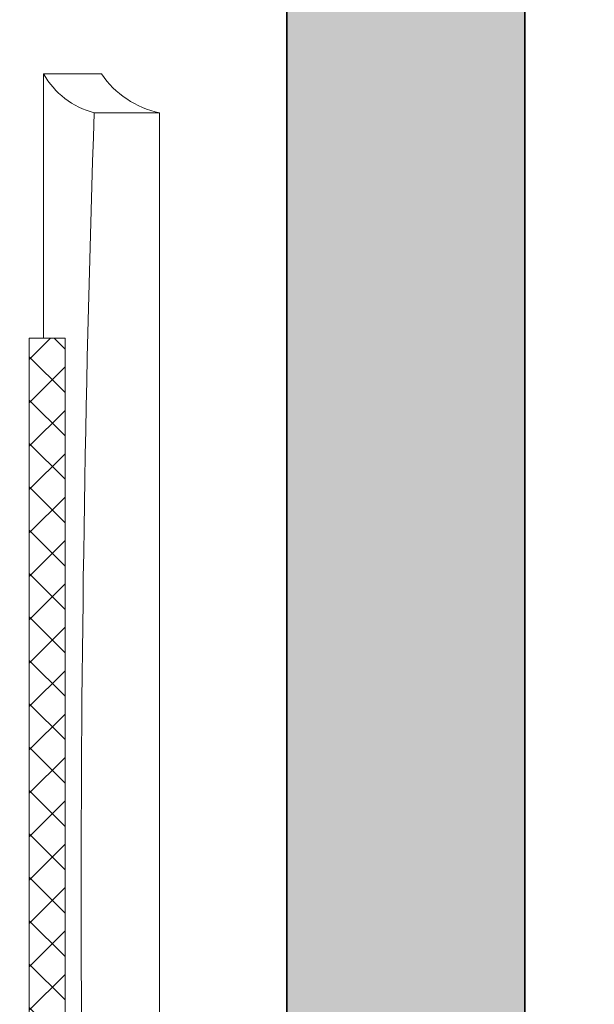
# Model space of a CAD drawing. Units: inches. Extents: x 2083 to 3317, y 1141 to 2115.
# Tile 243 of 256: x 3108 to 3130, y 1327 to 1365. Entities that reach past the tile are written whole.
import ezdxf

# ---------------------------------------------------------------- set-up
doc = ezdxf.new("R2010")
doc.units = ezdxf.units.IN
for name, color, linetype, lineweight in [('A-ANNO-DIMS', 2, 'Continuous', 18), ('A-FURN', 8, 'Continuous', 18), ('A-WALL', 7, 'Continuous', 35), ('www.cadblocksfree.com', 7, 'Continuous', 9)]:
    doc.layers.add(name, color=color, linetype=linetype, lineweight=lineweight)
doc.layers.add('A-WALL-PATT', color=251, linetype='Continuous', lineweight=13, true_color=0x636466)
doc.styles.get("Standard").update_dxf_attribs({"font": 'arial.ttf'})
doc.dimstyles.new('ISO-25', dxfattribs={"dimtxt": 12, "dimasz": 12, "dimexe": 1.25, "dimexo": 0.625, "dimtad": 1, "dimlunit": 3, "dimtxsty": 'Standard', "dimcen": 2.5, "dimadec": 0, "dimazin": 0, "dimtfac": 1, "dimtmove": 0, "dimatfit": 3, "dimfxl": 1, "dimarcsym": 0})

# ---------------------------------------------------------------- blocks, each defined once
blk = doc.blocks.new('bed')
at = {"layer": 'www.cadblocksfree.com', "ltscale": 0.2}
h = blk.add_hatch(dxfattribs=at)
h.set_pattern_fill('ANSI37,_O', color=256, scale=0.393701)
h.set_pattern_definition([(45, (2420.7222, -262.9689), (-0.8838835, 0.8838835), []), (135, (2420.7222, -262.9689), (-0.8838835, -0.8838835), [])])
h.paths.add_polyline_path([(3417.573, 1472.402), (3372.192, 1472.402), (3372.192, 1470.941), (3417.573, 1470.941)])
for p, q in [((3363.002, 1473.586), (3363.002, 1476.249)), ((3372.192, 1472.402), (3417.573, 1472.402)), ((3372.192, 1470.941), (3372.192, 1472.402)), ((3372.192, 1470.941), (3417.573, 1470.941))]:
    blk.add_line(p, q, dxfattribs=at)
for points in [[(3426.763, 1476.249), (3363.002, 1476.249)], [(3361.418, 1473.886), (3361.418, 1471.524), (3372.192, 1471.524)]]:
    blk.add_lwpolyline(points, dxfattribs=at)
for centre, radius, start, end in [((3359.334, 1476.997), 3.744, 303.8271, 348.4775), ((3359.844, 1474.373), 3.255, 298.9176, 345.9939), ((3394.883, 2431.358), 958.303, 268.093559, 271.906441)]:
    blk.add_arc(centre, radius, start, end, dxfattribs=at)
blk = doc.blocks.new('*D9')
at = {"layer": 'A-ANNO-DIMS', "color": 0, "lineweight": -2, "transparency": 16777216}
for p, q in [((3127.585, 1486.761), (3190.403, 1486.761)), ((3189.153, 1474.761), (3189.153, 1275.261)), ((3127.585, 1263.261), (3190.403, 1263.261))]:
    blk.add_line(p, q, dxfattribs=at)
at = {"layer": 'A-ANNO-DIMS', "color": 0, "transparency": 16777216}
for points in [[(3187.153, 1474.761), (3191.153, 1474.761), (3189.153, 1486.761)], [(3187.153, 1275.261), (3191.153, 1275.261), (3189.153, 1263.261)]]:
    blk.add_solid(points, dxfattribs=at)
at = {"layer": 'Defpoints', "color": 0, "transparency": 16777216}
for p in [(3126.96, 1486.761), (3126.96, 1263.261), (3189.153, 1263.261)]:
    blk.add_point(p, dxfattribs=at)
at = {"layer": 'A-ANNO-DIMS', "color": 0, "transparency": 16777216, "insert": (3182.401, 1375.011), "char_height": 12, "attachment_point": 5, "rotation": 90}
blk.add_mtext('18\'-7.5"', dxfattribs=at)
blk = doc.blocks.new('*D35')
at = {"layer": 'A-ANNO-DIMS', "color": 0, "lineweight": -2, "transparency": 16777216}
for p, q in [((3127.585, 2020.761), (3180.56, 2020.761)), ((3179.31, 1275.261), (3179.31, 2008.761)), ((3127.585, 1263.261), (3180.56, 1263.261))]:
    blk.add_line(p, q, dxfattribs=at)
at = {"layer": 'A-ANNO-DIMS', "color": 0, "transparency": 16777216}
for points in [[(3177.31, 2008.761), (3181.31, 2008.761), (3179.31, 2020.761)], [(3177.31, 1275.261), (3181.31, 1275.261), (3179.31, 1263.261)]]:
    blk.add_solid(points, dxfattribs=at)
at = {"layer": 'Defpoints', "color": 0, "transparency": 16777216}
for p in [(3126.96, 2020.761), (3179.31, 2020.761), (3126.96, 1263.261)]:
    blk.add_point(p, dxfattribs=at)
at = {"layer": 'A-ANNO-DIMS', "color": 0, "transparency": 16777216, "insert": (3172.476, 1642.011), "char_height": 12, "attachment_point": 5, "rotation": 90}
blk.add_mtext('63\'-1 1/2"', dxfattribs=at)

msp = doc.modelspace()

# ---------------------------------------------------------------- hatches: boundary and pattern name
at = {"layer": 'A-WALL-PATT'}
h = msp.add_hatch(color=256, dxfattribs=at)
h.dxf.hatch_style = 1
h.paths.add_polyline_path([(3126.96, 2020.761), (2748.96, 2020.761), (2604.96, 2020.761), (2226.96, 2020.761), (2226.96, 1702.761), (2466.96, 1702.761), (2466.96, 1582.761), (2418.96, 1582.761), (2418.96, 1477.761), (2226.96, 1477.761), (2226.96, 1263.261), (2544.96, 1263.261), (2544.96, 1411.761), (2604.96, 1411.761), (2685.96, 1411.761), (2685.96, 1420.761), (2604.96, 1420.761), (2604.96, 1573.761), (2604.96, 1702.761), (2604.96, 2011.761), (2748.96, 2011.761), (2748.96, 1702.761), (2862.96, 1702.761), (2862.96, 1621.761), (2871.96, 1621.761), (2871.96, 1702.761), (2883.96, 1702.761), (2883.96, 1706.939, -0.026459), (2883.96, 1711.761), (2757.96, 1711.761), (2757.96, 1807.761), (2787.96, 1807.761), (2787.96, 1812.261), (2757.96, 1812.261), (2757.96, 2011.761), (2877.96, 2011.761), (2877.96, 1812.261), (2847.96, 1812.261), (2847.96, 1807.761), (2889.836, 1807.761), (2889.836, 1812.261), (2882.46, 1812.261), (2882.46, 2011.761), (3117.96, 2011.761), (3117.96, 1812.261), (2937.836, 1812.261), (2937.836, 1807.761), (2995.71, 1807.761), (2995.71, 1796.118), (3000.21, 1796.118), (3000.21, 1807.761), (3117.96, 1807.761), (3117.96, 1711.761), (3000.21, 1711.761), (3000.21, 1760.118), (2998.573, 1760.118, -0.020711), (2995.71, 1760.118), (2995.71, 1711.761), (2931.96, 1711.761), (2931.96, 1702.761), (3126.96, 1702.761)])
h.paths.add_polyline_path([(2471.46, 2011.761), (2471.46, 1810.011), (2462.717, 1810.011), (2462.717, 1805.511), (2505.96, 1805.511), (2505.96, 1810.011), (2475.96, 1810.011), (2475.96, 2011.761), (2595.96, 2011.761), (2595.96, 1810.011), (2565.96, 1810.011), (2565.96, 1805.511), (2595.96, 1805.511), (2595.96, 1711.761), (2235.96, 1711.761), (2235.96, 1805.511), (2353.71, 1805.511), (2353.71, 1796.054), (2358.21, 1796.054), (2358.21, 1805.511), (2414.717, 1805.511), (2414.717, 1810.011), (2235.96, 1810.011), (2235.96, 2011.761)], flags=16)
h.paths.add_polyline_path([(2270.205, 1994.61), (2270.205, 1970.61), (2246.205, 1970.61), (2246.205, 1994.61)], flags=0)
edge = h.paths.add_edge_path(flags=0)
edge.add_ellipse((2332.027, 1899.798), major_axis=(-3.043, 3.043), ratio=0.168252, start_angle=-161.3322, end_angle=-156.3071, ccw=False)
edge.add_ellipse((2333.082, 1898.744), major_axis=(-1.055, 1.055), ratio=0.453532, start_angle=-123.371, end_angle=-94.1591)
edge = h.paths.add_edge_path(flags=0)
edge.add_ellipse((2332.027, 1968.876), major_axis=(3.043, 3.043), ratio=0.168252, start_angle=18.6678, end_angle=23.6929)
edge.add_spline(control_points=[(2332.926, 1970.691), (2332.227, 1970.336), (2330.894, 1969.659), (2328.413, 1970.932), (2327.204, 1967.749), (2324.71, 1969.956), (2322.533, 1967.012), (2320.013, 1971.296), (2317.68, 1968.158), (2316.041, 1967.102), (2315.427, 1966.81)], knot_values=[0, 0, 0, 0, 2.267059, 4.324559, 6.685584, 8.878641, 11.121502, 14.300359, 17.755284, 19.732645, 19.732645, 19.732645, 19.732645], degree=3, periodic=0)
edge.add_ellipse((2332.027, 1968.876), major_axis=(3.043, 3.043), ratio=0.168252, start_angle=18.6678, end_angle=23.6929, ccw=False)
edge.add_ellipse((2333.082, 1969.931), major_axis=(1.055, 1.055), ratio=0.453532, start_angle=56.629, end_angle=85.8409, ccw=False)
edge = h.paths.add_edge_path(flags=0)
edge.add_spline(control_points=[(2296.428, 1967.988), (2293.628, 1965.336), (2287.704, 1959.727), (2299.744, 1949.996), (2294.533, 1935.669), (2290.573, 1920.604), (2293.394, 1909.974), (2296.185, 1904.967)], knot_values=[0.099185, 0.099185, 0.099185, 0.099185, 0.345301, 0.619822, 0.982653, 1.386093, 1.810555, 1.810555, 1.810555, 1.810555], degree=3, periodic=0)
edge.add_spline(control_points=[(2296.185, 1904.967), (2297.384, 1902.619), (2298.001, 1901.949), (2298.553, 1901.468)], knot_values=[0.006246, 0.006246, 0.006246, 0.006246, 0.055476, 0.055476, 0.055476, 0.055476], degree=3, periodic=0)
edge.add_spline(control_points=[(2298.553, 1901.468), (2297.259, 1900.923), (2295.225, 1900.232), (2293.06, 1900.614), (2292.101, 1900.788), (2292.09, 1900.791)], knot_values=[0.312835, 0.312835, 0.312835, 0.312835, 0.40178, 0.474987, 0.475903, 0.475903, 0.475903, 0.475903], degree=3, periodic=0)
edge.add_arc((2292.794, 1904.664), 3.937, 215.4209, 259.6982, ccw=False)
edge.add_spline(control_points=[(2289.585, 1902.382), (2289.477, 1902.535), (2289.368, 1902.688), (2289.261, 1902.841)], knot_values=[0.102872, 0.102872, 0.102872, 0.102872, 0.116896, 0.116896, 0.116896, 0.116896], degree=3, periodic=0)
edge.add_spline(control_points=[(2289.261, 1902.841), (2288.687, 1902.55), (2287.64, 1902.02), (2285.881, 1901.874), (2283.853, 1901.504), (2281.72, 1899.711), (2278.467, 1899.493), (2276.157, 1901.883), (2272.259, 1899.804), (2267.778, 1901.843), (2262.244, 1900.184), (2257.415, 1901.782), (2254.318, 1900.726), (2253.178, 1900.337)], knot_values=[0, 0, 0, 0, 1.907977, 3.477176, 5.261074, 7.972851, 11.680248, 13.717921, 16.939592, 22.789562, 27.502503, 33.595215, 37.145618, 37.145618, 37.145618, 37.145618], degree=3, periodic=0)
edge.add_line((2253.178, 1900.337), (2250.244, 1902.841))
edge.add_line((2250.244, 1902.841), (2250.244, 1965.833))
edge.add_line((2250.244, 1965.833), (2253.178, 1968.337))
edge.add_spline(control_points=[(2253.178, 1968.337), (2254.318, 1967.948), (2257.415, 1966.892), (2262.244, 1968.49), (2267.778, 1966.831), (2271.527, 1968.537), (2273.876, 1967.828), (2274.207, 1967.728)], knot_values=[0, 0, 0, 0, 0.09018, 0.244935, 0.364644, 0.513233, 0.537855, 0.537855, 0.537855, 0.537855], degree=3, periodic=0)
edge.add_arc((2274.353, 1963.793), 3.937, 72.0511, 92.1279, ccw=False)
edge.add_arc((2281.297, 1985.23), 18.596, 252.0511, 288.5657)
edge.add_arc((2292.317, 1956.029), 12.646, 71.0268, 113.7782, ccw=False)
edge = h.paths.add_edge_path(flags=0)
edge.add_spline(control_points=[(2274.899, 1951.856), (2275.066, 1951.617), (2275.233, 1951.377), (2275.398, 1951.136)], knot_values=[1.409916, 1.409916, 1.409916, 1.409916, 1.43159, 1.43159, 1.43159, 1.43159], degree=3, periodic=0)
edge.add_spline(control_points=[(2275.398, 1951.136), (2275.792, 1950.562), (2276.179, 1949.984), (2276.546, 1949.397)], knot_values=[1.358238, 1.358238, 1.358238, 1.358238, 1.409916, 1.409916, 1.409916, 1.409916], degree=3, periodic=0)
edge.add_line((2276.546, 1949.397), (2277.437, 1947.862))
edge.add_spline(control_points=[(2277.437, 1947.862), (2276.304, 1945.673), (2274.64, 1942.427), (2274.632, 1938.094), (2272.799, 1930.852), (2274.356, 1943.897), (2275.948, 1947.923), (2276.546, 1949.397)], knot_values=[0.005632, 0.005632, 0.005632, 0.005632, 0.186014, 0.266002, 0.357087, 0.59639, 0.739732, 0.739732, 0.739732, 0.739732], degree=3, periodic=0)
edge.add_spline(control_points=[(2276.546, 1949.397), (2276.179, 1949.984), (2275.792, 1950.562), (2275.398, 1951.136)], knot_values=[1.358238, 1.358238, 1.358238, 1.358238, 1.409916, 1.409916, 1.409916, 1.409916], degree=3, periodic=0)
edge.add_spline(control_points=[(2275.398, 1951.136), (2274.943, 1950.08), (2274.208, 1948.025), (2273.935, 1944.851), (2272.469, 1937.627), (2273.466, 1945.696), (2274.701, 1951.059), (2274.899, 1951.856)], knot_values=[0.104364, 0.104364, 0.104364, 0.104364, 0.189636, 0.269624, 0.36071, 0.600013, 0.644622, 0.644622, 0.644622, 0.644622], degree=3, periodic=0)
h.paths.add_polyline_path([(2269.168, 1963.128, -0.357527), (2268.171, 1960.976, -0.092561), (2268.171, 1939.436, -0.357527), (2269.168, 1937.285, -0.357527), (2267.016, 1938.282, -0.164785), (2254.686, 1938.282, -0.357527), (2252.534, 1937.285, -0.357527), (2253.531, 1939.436, -0.092561), (2253.531, 1960.976, -0.357527), (2252.534, 1963.128, -0.357527), (2254.686, 1962.131, -0.164785), (2267.016, 1962.131, -0.357527)], flags=0)
h.paths.add_polyline_path([(2248.874, 1967.802), (2248.874, 1957.028), (2249.458, 1957.028), (2249.458, 1911.647), (2248.874, 1911.647), (2248.874, 1900.873), (2246.512, 1900.873, 0.197327), (2244.15, 1902.457), (2244.15, 1966.218, 0.197327), (2246.512, 1967.802)], flags=0)
h.paths.add_polyline_path([(2269.168, 1931.389, -0.357527), (2268.171, 1929.238, -0.092561), (2268.171, 1907.698, -0.357527), (2269.168, 1905.547, -0.357527), (2267.016, 1906.544, -0.164785), (2254.686, 1906.544, -0.357527), (2252.534, 1905.547, -0.357527), (2253.531, 1907.698, -0.092561), (2253.531, 1929.238, -0.357527), (2252.534, 1931.389, -0.357527), (2254.686, 1930.392, -0.164785), (2267.016, 1930.392, -0.357527)], flags=0)
edge = h.paths.add_edge_path(flags=0)
edge.add_spline(control_points=[(2276.197, 1906.724), (2276.168, 1909.029), (2276.114, 1913.372), (2270.598, 1924.925), (2273.905, 1919.013), (2275.922, 1916.262), (2275.475, 1912.402), (2277.258, 1910.381), (2276.696, 1908.225), (2276.646, 1906.813), (2276.618, 1906.008)], knot_values=[0, 0, 0, 0, 8.61026, 16.221274, 18.843057, 23.804898, 27.440828, 29.356102, 31.203478, 33.650687, 33.650687, 33.650687, 33.650687], degree=3, periodic=0)
edge.add_spline(control_points=[(2276.618, 1906.008), (2276.623, 1905.624), (2276.498, 1904.629), (2275.442, 1903.855), (2274.937, 1903.08), (2274.859, 1902.841)], knot_values=[0.156488, 0.156488, 0.156488, 0.156488, 0.184398, 0.231376, 0.250598, 0.250598, 0.250598, 0.250598], degree=3, periodic=0)
edge.add_line((2274.859, 1902.841), (2276.506, 1902.841))
edge.add_spline(control_points=[(2276.506, 1902.841), (2276.788, 1903.085), (2277.665, 1904.125), (2278.25, 1904.341), (2277.654, 1908.527), (2278.156, 1906.228), (2278.1, 1905.286), (2278.847, 1904.069), (2277.857, 1903.415), (2277.874, 1902.991), (2277.904, 1902.841)], knot_values=[0.059574, 0.059574, 0.059574, 0.059574, 0.080753, 0.103741, 0.16972, 0.176036, 0.207137, 0.240474, 0.262341, 0.27366, 0.27366, 0.27366, 0.27366], degree=3, periodic=0)
edge.add_line((2277.904, 1902.841), (2280.03, 1902.841))
edge.add_spline(control_points=[(2280.03, 1902.841), (2279.888, 1903.088), (2279.499, 1903.982), (2280.152, 1905.939), (2278.104, 1909.658), (2279.762, 1907.185), (2280.328, 1904.875), (2280.485, 1903.49), (2281.463, 1903.249), (2281.758, 1902.936), (2281.834, 1902.841)], knot_values=[0.013856, 0.013856, 0.013856, 0.013856, 0.034874, 0.088867, 0.107879, 0.126738, 0.158714, 0.193757, 0.217487, 0.226722, 0.226722, 0.226722, 0.226722], degree=3, periodic=0)
edge.add_spline(control_points=[(2281.834, 1902.841), (2281.788, 1902.827), (2281.647, 1902.783), (2281.396, 1902.859), (2281.088, 1902.985), (2280.721, 1903.061), (2280.333, 1903.026), (2280.125, 1902.899), (2280.03, 1902.841)], knot_values=[0, 0, 0, 0, 0.14413, 0.435517, 0.749276, 1.153046, 1.548371, 1.878348, 1.878348, 1.878348, 1.878348], degree=3, periodic=0)
edge.add_line((2280.03, 1902.841), (2277.904, 1902.841))
edge.add_spline(control_points=[(2277.904, 1902.841), (2277.893, 1902.796), (2277.865, 1902.68), (2277.607, 1902.687), (2277.274, 1902.801), (2276.838, 1902.62), (2276.584, 1902.789), (2276.506, 1902.841)], knot_values=[0, 0, 0, 0, 0.127189, 0.326199, 0.628009, 1.24357, 1.515331, 1.515331, 1.515331, 1.515331], degree=3, periodic=0)
edge.add_line((2276.506, 1902.841), (2274.859, 1902.841))
edge.add_spline(control_points=[(2274.859, 1902.841), (2274.814, 1902.899), (2274.725, 1903.013), (2274.493, 1903.119), (2274.244, 1902.961), (2273.937, 1903.185), (2273.614, 1902.983), (2273.408, 1902.883), (2273.322, 1902.841)], knot_values=[0, 0, 0, 0, 0.21843, 0.436957, 0.687977, 0.990379, 1.398396, 1.69185, 1.69185, 1.69185, 1.69185], degree=3, periodic=0)
edge.add_spline(control_points=[(2273.322, 1902.841), (2273.617, 1903.446), (2274.274, 1904.538), (2276.027, 1904.574), (2276.207, 1906.584), (2276.197, 1906.724)], knot_values=[0.012227, 0.012227, 0.012227, 0.012227, 0.059472, 0.106218, 0.134458, 0.134458, 0.134458, 0.134458], degree=3, periodic=0)
h.paths.add_polyline_path([(2270.776, 1897.79), (2270.776, 1873.79), (2246.776, 1873.79), (2246.776, 1897.79)], flags=0)
h.paths.add_polyline_path([(2353.71, 1760.005), (2353.71, 1760.054), (2358.21, 1760.054, -0.033729)], flags=0)
h.paths.add_polyline_path([(2321.819, 1737.529), (2341.995, 1737.529, -0.414214), (2343.203, 1736.321), (2343.203, 1721.021, -0.414214), (2341.995, 1719.813), (2321.819, 1719.813, -0.414214), (2320.611, 1721.021), (2320.611, 1736.321, -0.414214)], flags=0)
h.paths.add_polyline_path([(2324.235, 1736.321), (2339.579, 1736.321, -0.414214), (2341.995, 1733.905), (2341.995, 1725.45, -0.414214), (2339.579, 1723.034), (2333.681, 1723.034), (2333.845, 1722.045, -0.870646), (2335.425, 1721.826, -0.767327), (2333.923, 1721.423), (2331.291, 1721.423, -0.767327), (2329.788, 1721.826, -0.870646), (2331.368, 1722.045), (2331.533, 1723.034), (2324.235, 1723.034, -0.414214), (2321.819, 1725.45), (2321.819, 1733.905, -0.414214)], flags=0)
h.paths.add_polyline_path([(2570.484, 1928.615), (2589.684, 1928.615), (2590.169, 1928.615), (2590.169, 1904.993), (2570.484, 1904.993)], flags=0)
h.paths.add_polyline_path([(2574.447, 1927.264, -1), (2572.829, 1927.264, -1)], flags=0)
h.paths.add_polyline_path([(2573.09, 1926.941), (2573.925, 1927.776), (2574.148, 1927.553), (2573.313, 1926.718)], flags=0)
h.paths.add_polyline_path([(2578.779, 1919.73, -1), (2571.592, 1919.73, -1)], flags=0)
h.paths.add_polyline_path([(2578.385, 1919.73, -1), (2571.985, 1919.73, -1)], flags=0)
h.paths.add_polyline_path([(2331.596, 1729.476, -1), (2333.618, 1729.476, -1)], flags=0)
h.paths.add_polyline_path([(2578.034, 1927.264, -1), (2576.416, 1927.264, -1)], flags=0)
h.paths.add_polyline_path([(2576.689, 1927.531), (2576.912, 1927.754), (2577.747, 1926.919), (2577.524, 1926.696)], flags=0)
h.paths.add_polyline_path([(2578.139, 1909.86, -1), (2572.232, 1909.86, -1)], flags=0)
h.paths.add_polyline_path([(2577.745, 1909.86, -1), (2572.625, 1909.86, -1)], flags=0)
h.paths.add_polyline_path([(2583.798, 1927.264, -1), (2582.179, 1927.264, -1)], flags=0)
h.paths.add_polyline_path([(2582.719, 1927.754), (2583.554, 1926.919), (2583.331, 1926.696), (2582.496, 1927.531)], flags=0)
h.paths.add_polyline_path([(2582.496, 1927.531), (2582.719, 1927.754), (2583.554, 1926.919), (2583.331, 1926.696)], flags=0)
h.paths.add_polyline_path([(2587.739, 1920.53, -1), (2581.832, 1920.53, -1)], flags=0)
h.paths.add_polyline_path([(2587.345, 1920.53, -1), (2582.225, 1920.53, -1)], flags=0)
h.paths.add_polyline_path([(2587.385, 1927.264, -1), (2585.766, 1927.264, -1)], flags=0)
h.paths.add_polyline_path([(2586.082, 1926.98), (2586.917, 1927.815), (2587.14, 1927.593), (2586.305, 1926.758)], flags=0)
h.paths.add_polyline_path([(2588.379, 1910.66, -1), (2581.192, 1910.66, -1)], flags=0)
h.paths.add_polyline_path([(2587.985, 1910.66, -1), (2581.585, 1910.66, -1)], flags=0)
h.paths.add_polyline_path([(2417.168, 1729.478), (2437.344, 1729.478, -0.414214), (2438.552, 1728.27), (2438.552, 1712.969, -0.414214), (2437.344, 1711.761), (2417.168, 1711.761, -0.414214), (2415.96, 1712.969), (2415.96, 1728.27, -0.414214)], flags=0)
h.paths.add_polyline_path([(2419.584, 1728.27), (2434.928, 1728.27, -0.414214), (2437.344, 1725.854), (2437.344, 1717.398, -0.414214), (2434.928, 1714.983), (2429.029, 1714.983), (2429.194, 1713.994, -0.870646), (2430.774, 1713.775, -0.767327), (2429.271, 1713.372), (2426.64, 1713.372, -0.767327), (2425.137, 1713.775, -0.870646), (2426.717, 1713.994), (2426.882, 1714.983), (2419.584, 1714.983, -0.414214), (2417.168, 1717.398), (2417.168, 1725.854, -0.414214)], flags=0)
h.paths.add_polyline_path([(2419.584, 1728.27), (2434.928, 1728.27, -0.414214), (2437.344, 1725.854), (2437.344, 1717.398, -0.414214), (2434.928, 1714.983), (2429.029, 1714.983), (2428.358, 1719.009), (2427.553, 1719.009), (2426.882, 1714.983), (2419.584, 1714.983, -0.414214), (2417.168, 1717.398), (2417.168, 1725.854, -0.414214)], flags=0)
h.paths.add_polyline_path([(2426.944, 1721.425, -1), (2428.967, 1721.425, -1)], flags=0)
h.paths.add_polyline_path([(2475.96, 1702.761), (2595.96, 1702.761), (2595.96, 1582.761), (2475.96, 1582.761)], flags=16)
h.paths.add_polyline_path([(2427.96, 1573.761), (2595.96, 1573.761), (2595.96, 1468.761), (2595.96, 1420.761), (2384.46, 1420.761), (2384.46, 1468.761), (2427.96, 1468.761)], flags=16)
h.paths.add_polyline_path([(2379.96, 1468.761), (2379.96, 1420.761), (2235.96, 1420.761), (2235.96, 1468.761)], flags=16)
h.paths.add_polyline_path([(2317.816, 1466.696), (2337.992, 1466.696, -0.414214), (2339.2, 1465.488), (2339.2, 1450.187, -0.414214), (2337.992, 1448.979), (2317.816, 1448.979, -0.414214), (2316.608, 1450.187), (2316.608, 1465.488, -0.414214)], flags=0)
h.paths.add_polyline_path([(2320.232, 1465.488), (2335.576, 1465.488, -0.414214), (2337.992, 1463.072), (2337.992, 1454.616, -0.414214), (2335.576, 1452.2), (2329.677, 1452.2), (2329.842, 1451.212, -0.870646), (2331.422, 1450.992, -0.767327), (2329.92, 1450.59), (2327.288, 1450.59, -0.767327), (2325.785, 1450.992, -0.870646), (2327.365, 1451.212), (2327.53, 1452.2), (2320.232, 1452.2, -0.414214), (2317.816, 1454.616), (2317.816, 1463.072, -0.414214)], flags=0)
h.paths.add_polyline_path([(2320.232, 1465.488), (2335.576, 1465.488, -0.414214), (2337.992, 1463.072), (2337.992, 1454.616, -0.414214), (2335.576, 1452.2), (2329.677, 1452.2), (2329.006, 1456.227), (2328.201, 1456.227), (2327.53, 1452.2), (2320.232, 1452.2, -0.414214), (2317.816, 1454.616), (2317.816, 1463.072, -0.414214)], flags=0)
h.paths.add_polyline_path([(2327.593, 1458.643, -1), (2329.615, 1458.643, -1)], flags=0)
h.paths.add_polyline_path([(2244.412, 1433.34), (2241.921, 1433.34, -0.414214), (2240.018, 1435.244), (2240.018, 1440.953, -0.414211), (2241.921, 1442.856), (2244.412, 1442.856, -1.976472)], flags=0)
h.paths.add_polyline_path([(2245.357, 1434.398, -0.414214), (2245.357, 1441.799, -2.144098)], flags=0)
h.paths.add_polyline_path([(2535.96, 1416.261), (2535.96, 1272.261), (2235.96, 1272.261), (2235.96, 1416.261)], flags=16)
h.paths.add_polyline_path([(2260.12, 1384.293), (2260.12, 1362.039), (2237.865, 1362.039), (2237.865, 1384.293)], flags=0)
edge = h.paths.add_edge_path(flags=0)
edge.add_line((2318.252, 1362.093), (2318.146, 1362.001))
edge.add_ellipse((2317.445, 1360.431), major_axis=(2.822, 2.822), ratio=0.168252, start_angle=18.6678, end_angle=20.9481, ccw=False)
edge.add_ellipse((2318.423, 1361.409), major_axis=(0.978, 0.978), ratio=0.453532, start_angle=56.629, end_angle=70.2262, ccw=False)
edge = h.paths.add_edge_path(flags=0)
edge.add_line((2319.107, 1295.571), (2319.015, 1295.677))
edge.add_ellipse((2317.445, 1296.378), major_axis=(-2.822, 2.822), ratio=0.168252, start_angle=-161.3322, end_angle=-159.0519, ccw=False)
edge.add_ellipse((2318.423, 1295.4), major_axis=(-0.978, 0.978), ratio=0.453532, start_angle=-123.371, end_angle=-109.7738)
edge = h.paths.add_edge_path(flags=0)
edge.add_spline(control_points=[(2284.21, 1301.17), (2284.581, 1300.445), (2284.891, 1299.892), (2285.16, 1299.461)], knot_values=[0.039066, 0.039066, 0.039066, 0.039066, 0.055476, 0.055476, 0.055476, 0.055476], degree=3, periodic=0)
edge.add_line((2285.16, 1299.461), (2284.21, 1301.17))
edge = h.paths.add_edge_path(flags=0)
edge.add_line((2280.412, 1297.298), (2283.37, 1297.036))
edge.add_line((2283.37, 1297.036), (2286.406, 1297.926))
edge.add_spline(control_points=[(2286.406, 1297.926), (2285.305, 1297.463), (2284.345, 1297.129), (2283.37, 1297.036)], knot_values=[0.394369, 0.394369, 0.394369, 0.394369, 0.475903, 0.475903, 0.475903, 0.475903], degree=3, periodic=0)
edge.add_spline(control_points=[(2283.37, 1297.036), (2283.281, 1297.028), (2282.316, 1296.957), (2281.313, 1297.134), (2280.423, 1297.296), (2280.412, 1297.298)], knot_values=[0.312835, 0.312835, 0.312835, 0.312835, 0.320246, 0.393453, 0.394369, 0.394369, 0.394369, 0.394369], degree=3, periodic=0)
edge = h.paths.add_edge_path(flags=0)
edge.add_line((2284.436, 1359.607), (2280.446, 1355.328))
edge.add_line((2280.446, 1355.328), (2279.58, 1351.018))
edge.add_line((2279.58, 1351.018), (2282.413, 1346.58))
edge.add_spline(control_points=[(2282.413, 1346.58), (2283.153, 1345.589), (2284.253, 1344.029), (2284.801, 1342.387), (2284.935, 1341.806)], knot_values=[1.240098, 1.240098, 1.240098, 1.240098, 1.332892, 1.382712, 1.382712, 1.382712, 1.382712], degree=3, periodic=0)
edge.add_spline(control_points=[(2284.935, 1341.806), (2285.319, 1340.141), (2285.233, 1338.409), (2284.91, 1336.654)], knot_values=[1.097484, 1.097484, 1.097484, 1.097484, 1.240098, 1.240098, 1.240098, 1.240098], degree=3, periodic=0)
edge.add_spline(control_points=[(2284.91, 1336.654), (2284.587, 1334.899), (2284.027, 1333.12), (2283.463, 1331.361)], knot_values=[0.95487, 0.95487, 0.95487, 0.95487, 1.097484, 1.097484, 1.097484, 1.097484], degree=3, periodic=0)
edge.add_line((2283.463, 1331.361), (2281.89, 1326.153))
edge.add_line((2281.89, 1326.153), (2280.756, 1321.056))
edge.add_line((2280.756, 1321.056), (2280.299, 1316.002))
edge.add_line((2280.299, 1316.002), (2280.716, 1310.95))
edge.add_line((2280.716, 1310.95), (2282.028, 1305.972))
edge.add_line((2282.028, 1305.972), (2284.21, 1301.17))
edge.add_spline(control_points=[(2284.21, 1301.17), (2283.341, 1302.73), (2282.612, 1304.336), (2282.028, 1305.972)], knot_values=[0.099185, 0.099185, 0.099185, 0.099185, 0.241799, 0.241799, 0.241799, 0.241799], degree=3, periodic=0)
edge.add_spline(control_points=[(2282.028, 1305.972), (2281.444, 1307.608), (2281.005, 1309.273), (2280.716, 1310.95)], knot_values=[0.241799, 0.241799, 0.241799, 0.241799, 0.384413, 0.384413, 0.384413, 0.384413], degree=3, periodic=0)
edge.add_spline(control_points=[(2280.716, 1310.95), (2280.433, 1312.588), (2280.289, 1314.277), (2280.299, 1315.962), (2280.299, 1316.002)], knot_values=[0.384413, 0.384413, 0.384413, 0.384413, 0.523647, 0.527028, 0.527028, 0.527028, 0.527028], degree=3, periodic=0)
edge.add_spline(control_points=[(2280.299, 1316.002), (2280.312, 1317.687), (2280.478, 1319.368), (2280.756, 1321.056)], knot_values=[0.527028, 0.527028, 0.527028, 0.527028, 0.669642, 0.669642, 0.669642, 0.669642], degree=3, periodic=0)
edge.add_spline(control_points=[(2280.756, 1321.056), (2281.035, 1322.744), (2281.426, 1324.44), (2281.89, 1326.153)], knot_values=[0.669642, 0.669642, 0.669642, 0.669642, 0.812256, 0.812256, 0.812256, 0.812256], degree=3, periodic=0)
edge.add_spline(control_points=[(2281.89, 1326.153), (2282.264, 1327.533), (2282.788, 1329.262), (2283.353, 1331.018), (2283.463, 1331.361)], knot_values=[0.812256, 0.812256, 0.812256, 0.812256, 0.927087, 0.95487, 0.95487, 0.95487, 0.95487], degree=3, periodic=0)
edge.add_line((2283.463, 1331.361), (2284.91, 1336.654))
edge.add_line((2284.91, 1336.654), (2284.935, 1341.806))
edge.add_line((2284.935, 1341.806), (2282.413, 1346.58))
edge.add_spline(control_points=[(2282.413, 1346.58), (2281.275, 1348.104), (2280.078, 1349.57), (2279.58, 1351.018)], knot_values=[1.382712, 1.382712, 1.382712, 1.382712, 1.525326, 1.525326, 1.525326, 1.525326], degree=3, periodic=0)
edge.add_spline(control_points=[(2279.58, 1351.018), (2279.443, 1351.415), (2279.136, 1352.857), (2279.735, 1354.29), (2280.446, 1355.328)], knot_values=[1.525326, 1.525326, 1.525326, 1.525326, 1.564439, 1.667941, 1.667941, 1.667941, 1.667941], degree=3, periodic=0)
edge.add_spline(control_points=[(2280.446, 1355.328), (2281.426, 1356.758), (2282.931, 1358.183), (2284.436, 1359.607)], knot_values=[1.667941, 1.667941, 1.667941, 1.667941, 1.810555, 1.810555, 1.810555, 1.810555], degree=3, periodic=0)
edge.add_arc((2280.623, 1348.518), 11.726, 71.0268, 113.7782)
edge.add_arc((2270.405, 1375.595), 17.244, 252.0511, 288.5657, ccw=False)
edge.add_arc((2263.966, 1355.718), 3.651, 72.0511, 92.1279)
edge.add_arc((2263.966, 1355.718), 3.651, 92.1279, 177.9851)
edge.add_spline(control_points=[(2260.318, 1355.846), (2260.26, 1354.221), (2260.551, 1350.187), (2262.999, 1346.766), (2264.473, 1344.649)], knot_values=[1.43159, 1.43159, 1.43159, 1.43159, 1.564144, 1.770695, 1.770695, 1.770695, 1.770695], degree=3, periodic=0)
edge.add_line((2264.473, 1344.649), (2264.936, 1343.983))
edge.add_spline(control_points=[(2263.801, 1340.248), (2263.843, 1340.514), (2264.067, 1341.756), (2264.513, 1343.002), (2264.935, 1343.981)], knot_values=[0.53657, 0.53657, 0.53657, 0.53657, 0.559349, 0.644622, 0.644622, 0.644622, 0.644622], degree=3, periodic=0)
edge.add_spline(control_points=[(2264.935, 1343.981), (2265.118, 1343.715), (2265.299, 1343.448), (2265.477, 1343.179)], knot_values=[1.384077, 1.384077, 1.384077, 1.384077, 1.409916, 1.409916, 1.409916, 1.409916], degree=3, periodic=0)
edge.add_spline(control_points=[(2265.477, 1343.179), (2265.655, 1342.911), (2265.829, 1342.641), (2265.999, 1342.369)], knot_values=[1.358238, 1.358238, 1.358238, 1.358238, 1.384077, 1.384077, 1.384077, 1.384077], degree=3, periodic=0)
edge.add_line((2265.999, 1342.369), (2266.826, 1340.946))
edge.add_spline(control_points=[(2266.826, 1340.946), (2268.894, 1337.09), (2271.398, 1325.843), (2270.516, 1310.569), (2275.919, 1301.861), (2277.79, 1299.199)], knot_values=[0.116896, 0.116896, 0.116896, 0.116896, 0.472987, 1.050969, 1.313793, 1.313793, 1.313793, 1.313793], degree=3, periodic=0)
edge.add_spline(control_points=[(2277.79, 1299.199), (2277.839, 1299.128), (2277.889, 1299.057), (2277.94, 1298.987)], knot_values=[0.109884, 0.109884, 0.109884, 0.109884, 0.116896, 0.116896, 0.116896, 0.116896], degree=3, periodic=0)
edge.add_line((2277.94, 1298.987), (2277.789, 1299.199))
edge.add_spline(control_points=[(2277.789, 1299.199), (2277.257, 1298.929), (2276.286, 1298.438), (2275.039, 1298.334), (2274.383, 1298.239), (2274.215, 1298.209)], knot_values=[33.12187, 33.12187, 33.12187, 33.12187, 35.029056, 36.598255, 37.144827, 37.144827, 37.144827, 37.144827], degree=3, periodic=0)
edge.add_line((2274.215, 1298.209), (2273.073, 1297.893))
edge.add_spline(control_points=[(2273.073, 1297.893), (2272.323, 1297.58), (2271.039, 1296.511), (2269.248, 1296.226), (2268.423, 1296.375)], knot_values=[26.532584, 26.532584, 26.532584, 26.532584, 29.198919, 31.839101, 31.839101, 31.839101, 31.839101], degree=3, periodic=0)
edge.add_line((2268.423, 1296.375), (2263.879, 1297.458))
edge.add_spline(control_points=[(2263.879, 1297.458), (2263.556, 1297.359), (2261.86, 1296.839), (2260.239, 1297.282), (2258.933, 1297.516)], knot_values=[15.919551, 15.919551, 15.919551, 15.919551, 16.939592, 21.226067, 21.226067, 21.226067, 21.226067], degree=3, periodic=0)
edge.add_line((2258.933, 1297.516), (2254.055, 1297.329))
edge.add_spline(control_points=[(2254.055, 1297.329), (2253.756, 1297.296), (2252.114, 1297.165), (2250.462, 1297.544), (2249.13, 1297.668)], knot_values=[5.306517, 5.306517, 5.306517, 5.306517, 6.276435, 10.613034, 10.613034, 10.613034, 10.613034], degree=3, periodic=0)
edge.add_line((2249.13, 1297.668), (2244.332, 1296.878))
edge.add_line((2244.332, 1296.878), (2241.611, 1299.199))
edge.add_line((2241.611, 1299.199), (2241.611, 1357.609))
edge.add_line((2241.611, 1357.609), (2244.332, 1359.931))
edge.add_line((2244.332, 1359.931), (2252.729, 1359.543))
edge.add_spline(control_points=[(2252.729, 1359.543), (2252.871, 1359.546), (2253.306, 1359.548), (2253.74, 1359.514), (2254.032, 1359.482)], knot_values=[0.233291, 0.233291, 0.233291, 0.233291, 0.244935, 0.268927, 0.268927, 0.268927, 0.268927], degree=3, periodic=0)
edge.add_line((2254.032, 1359.482), (2259.587, 1359.416))
edge.add_spline(control_points=[(2259.587, 1359.416), (2260.677, 1359.629), (2262.073, 1359.897), (2263.524, 1359.459), (2263.83, 1359.366)], knot_values=[0.422516, 0.422516, 0.422516, 0.422516, 0.513233, 0.537855, 0.537855, 0.537855, 0.537855], degree=3, periodic=0)
edge.add_arc((2263.966, 1355.718), 3.651, 72.0511, 92.1279, ccw=False)
edge.add_arc((2270.405, 1375.595), 17.244, 252.0511, 288.5657)
edge.add_arc((2280.623, 1348.518), 11.726, 71.0268, 113.7782, ccw=False)
h.paths.add_polyline_path([(2240.341, 1359.435), (2240.341, 1349.444), (2240.882, 1349.444), (2240.882, 1307.365), (2240.341, 1307.365), (2240.341, 1297.374), (2238.15, 1297.374, 0.197327), (2235.96, 1298.843), (2235.96, 1357.966, 0.197327), (2238.15, 1359.435)], flags=0)
h.paths.add_polyline_path([(2259.158, 1355.101, -0.357527), (2258.233, 1353.106, -0.092561), (2258.233, 1333.133, -0.357527), (2259.158, 1331.138, -0.357527), (2257.163, 1332.062, -0.164785), (2245.729, 1332.062, -0.357527), (2243.735, 1331.138, -0.357527), (2244.659, 1333.133, -0.092561), (2244.659, 1353.106, -0.357527), (2243.735, 1355.101, -0.357527), (2245.729, 1354.176, -0.164785), (2257.163, 1354.176, -0.357527)], flags=0)
edge = h.paths.add_edge_path(flags=0)
edge.add_line((2265.999, 1342.369), (2266.826, 1340.946))
edge.add_line((2266.826, 1340.946), (2265.308, 1337.814))
edge.add_line((2265.308, 1337.814), (2264.358, 1334.653))
edge.add_line((2264.358, 1334.653), (2264.262, 1333.8))
edge.add_spline(control_points=[(2264.262, 1333.8), (2264.208, 1333.187), (2264.162, 1332.366), (2264.007, 1331.414), (2263.969, 1331.202)], knot_values=[0.464444, 0.464444, 0.464444, 0.464444, 0.516691, 0.531608, 0.531608, 0.531608, 0.531608], degree=3, periodic=0)
edge.add_spline(control_points=[(2263.969, 1331.202), (2263.775, 1330.119), (2263.424, 1328.791), (2263.257, 1328.531), (2263.234, 1328.515)], knot_values=[0.372682, 0.372682, 0.372682, 0.372682, 0.44885, 0.464444, 0.464444, 0.464444, 0.464444], degree=3, periodic=0)
edge.add_spline(control_points=[(2263.234, 1328.515), (2263.096, 1328.42), (2263.131, 1329.301), (2263.275, 1330.616)], knot_values=[0.280919, 0.280919, 0.280919, 0.280919, 0.372682, 0.372682, 0.372682, 0.372682], degree=3, periodic=0)
edge.add_spline(control_points=[(2263.275, 1330.616), (2263.419, 1331.93), (2263.672, 1333.677), (2263.97, 1335.315)], knot_values=[0.189157, 0.189157, 0.189157, 0.189157, 0.280919, 0.280919, 0.280919, 0.280919], degree=3, periodic=0)
edge.add_spline(control_points=[(2263.97, 1335.315), (2264.1, 1336.032), (2264.419, 1337.622), (2264.755, 1338.864), (2264.947, 1339.491)], knot_values=[0.097394, 0.097394, 0.097394, 0.097394, 0.137578, 0.189157, 0.189157, 0.189157, 0.189157], degree=3, periodic=0)
edge.add_spline(control_points=[(2264.947, 1339.491), (2265.29, 1340.606), (2265.644, 1341.494), (2265.999, 1342.369)], knot_values=[0.005632, 0.005632, 0.005632, 0.005632, 0.097394, 0.097394, 0.097394, 0.097394], degree=3, periodic=0)
h.paths.add_polyline_path([(2259.158, 1325.671, -0.357527), (2258.233, 1323.676, -0.092561), (2258.233, 1303.703, -0.357527), (2259.158, 1301.708, -0.357527), (2257.163, 1302.633, -0.164785), (2245.729, 1302.633, -0.357527), (2243.735, 1301.708, -0.357527), (2244.659, 1303.703, -0.092561), (2244.659, 1323.676, -0.357527), (2243.735, 1325.671, -0.357527), (2245.729, 1324.747, -0.164785), (2257.163, 1324.747, -0.357527)], flags=0)
edge = h.paths.add_edge_path(flags=0)
edge.add_spline(control_points=[(2261.709, 1317.311), (2261.679, 1317.418), (2261.762, 1317.389), (2262.491, 1316.09), (2262.962, 1315.301)], knot_values=[14.955861, 14.955861, 14.955861, 14.955861, 16.221274, 18.694826, 18.694826, 18.694826, 18.694826], degree=3, periodic=0)
edge.add_spline(control_points=[(2262.962, 1315.301), (2262.99, 1315.254), (2263.702, 1314.067), (2264.349, 1313.127), (2264.73, 1312.164)], knot_values=[18.694826, 18.694826, 18.694826, 18.694826, 18.843057, 22.433791, 22.433791, 22.433791, 22.433791], degree=3, periodic=0)
edge.add_spline(control_points=[(2264.73, 1312.164), (2264.876, 1311.796), (2265.177, 1310.77), (2265.143, 1309.559), (2265.248, 1308.824)], knot_values=[22.433791, 22.433791, 22.433791, 22.433791, 23.804898, 26.172756, 26.172756, 26.172756, 26.172756], degree=3, periodic=0)
edge.add_line((2265.248, 1308.824), (2265.851, 1307.172))
edge.add_spline(control_points=[(2265.851, 1307.172), (2266.065, 1306.822), (2266.384, 1306.332), (2266.424, 1305.781), (2266.42, 1305.611)], knot_values=[28.062562, 28.062562, 28.062562, 28.062562, 29.356102, 29.911721, 29.911721, 29.911721, 29.911721], degree=3, periodic=0)
edge.add_spline(control_points=[(2266.42, 1305.611), (2266.416, 1305.433), (2266.394, 1305.25), (2266.365, 1305.066)], knot_values=[29.911721, 29.911721, 29.911721, 29.911721, 30.497837, 30.497837, 30.497837, 30.497837], degree=3, periodic=0)
edge.add_line((2266.365, 1305.066), (2266.066, 1302.136))
edge.add_spline(control_points=[(2266.066, 1302.136), (2266.071, 1301.78), (2265.998, 1301.2), (2265.663, 1300.759), (2265.509, 1300.586)], knot_values=[0.156488, 0.156488, 0.156488, 0.156488, 0.184398, 0.203543, 0.203543, 0.203543, 0.203543], degree=3, periodic=0)
edge.add_line((2265.509, 1300.586), (2264.435, 1299.199))
edge.add_line((2264.435, 1299.199), (2265.962, 1299.199))
edge.add_line((2265.962, 1299.199), (2267.336, 1301.175))
edge.add_line((2267.336, 1301.175), (2267.312, 1301.986))
edge.add_spline(control_points=[(2267.312, 1301.986), (2267.261, 1302.862), (2267.16, 1303.737), (2267.271, 1303.326)], knot_values=[0.126229, 0.126229, 0.126229, 0.126229, 0.166617, 0.166617, 0.166617, 0.166617], degree=3, periodic=0)
edge.add_spline(control_points=[(2267.271, 1303.326), (2267.28, 1303.294), (2267.31, 1303.175), (2267.373, 1302.884), (2267.406, 1302.683), (2267.418, 1302.601)], knot_values=[0.166617, 0.166617, 0.166617, 0.166617, 0.16972, 0.176036, 0.180765, 0.180765, 0.180765, 0.180765], degree=3, periodic=0)
edge.add_spline(control_points=[(2267.744, 1300.988), (2267.688, 1301.151), (2267.481, 1301.657), (2267.484, 1302.145), (2267.418, 1302.601)], knot_values=[0.180765, 0.180765, 0.180765, 0.180765, 0.193767, 0.220139, 0.220139, 0.220139, 0.220139], degree=3, periodic=0)
edge.add_line((2267.418, 1302.601), (2267.744, 1300.988))
edge.add_spline(control_points=[(2267.744, 1300.988), (2267.832, 1300.732), (2267.932, 1300.31), (2267.555, 1299.975), (2267.429, 1299.829)], knot_values=[0.220139, 0.220139, 0.220139, 0.220139, 0.240474, 0.25489, 0.25489, 0.25489, 0.25489], degree=3, periodic=0)
edge.add_line((2267.429, 1299.829), (2267.258, 1299.199))
edge.add_line((2267.258, 1299.199), (2269.23, 1299.199))
edge.add_spline(control_points=[(2269.23, 1299.199), (2269.099, 1299.429), (2268.843, 1300.016), (2269.012, 1300.916), (2268.947, 1301.661)], knot_values=[0.013856, 0.013856, 0.013856, 0.013856, 0.034874, 0.067073, 0.067073, 0.067073, 0.067073], degree=3, periodic=0)
edge.add_line((2268.947, 1301.661), (2268.432, 1303.603))
edge.add_spline(control_points=[(2268.432, 1303.603), (2268.176, 1304.192), (2267.596, 1305.251), (2268.041, 1304.623), (2268.251, 1304.282)], knot_values=[0.090155, 0.090155, 0.090155, 0.090155, 0.107879, 0.120289, 0.120289, 0.120289, 0.120289], degree=3, periodic=0)
edge.add_spline(control_points=[(2268.251, 1304.282), (2268.361, 1304.105), (2269.058, 1302.918), (2269.383, 1301.59), (2269.521, 1300.776), (2269.575, 1300.556)], knot_values=[0.120289, 0.120289, 0.120289, 0.120289, 0.126738, 0.158714, 0.173506, 0.173506, 0.173506, 0.173506], degree=3, periodic=0)
edge.add_line((2269.575, 1300.556), (2270.686, 1299.421))
edge.add_spline(control_points=[(2270.686, 1299.421), (2270.767, 1299.357), (2270.838, 1299.281), (2270.903, 1299.199)], knot_values=[0.21816, 0.21816, 0.21816, 0.21816, 0.226722, 0.226722, 0.226722, 0.226722], degree=3, periodic=0)
edge.add_line((2270.937, 1299.193), (2270.903, 1299.199))
edge.add_spline(control_points=[(2270.903, 1299.199), (2270.86, 1299.186), (2270.73, 1299.146), (2270.496, 1299.216), (2270.272, 1299.308), (2270.121, 1299.348), (2270.063, 1299.36)], knot_values=[0.939174, 0.939174, 0.939174, 0.939174, 1.083304, 1.374691, 1.68845, 1.878348, 1.878348, 1.878348, 1.878348], degree=3, periodic=0)
edge.add_line((2270.063, 1299.36), (2269.23, 1299.199))
edge.add_line((2269.23, 1299.199), (2267.258, 1299.199))
edge.add_spline(control_points=[(2267.258, 1299.199), (2267.248, 1299.157), (2267.223, 1299.05), (2266.984, 1299.057), (2266.809, 1299.116), (2266.677, 1299.109), (2266.637, 1299.105)], knot_values=[0.757665, 0.757665, 0.757665, 0.757665, 0.884854, 1.083864, 1.385675, 1.515331, 1.515331, 1.515331, 1.515331], degree=3, periodic=0)
edge.add_spline(control_points=[(2266.637, 1299.105), (2266.485, 1299.089), (2266.236, 1299.017), (2266.035, 1299.151), (2265.962, 1299.199)], knot_values=[0, 0, 0, 0, 0.485905, 0.757665, 0.757665, 0.757665, 0.757665], degree=3, periodic=0)
edge.add_line((2265.962, 1299.199), (2264.435, 1299.199))
edge.add_line((2264.435, 1299.199), (2263.858, 1299.367))
edge.add_spline(control_points=[(2263.858, 1299.367), (2263.819, 1299.371), (2263.78, 1299.386), (2263.74, 1299.402)], knot_values=[0.845925, 0.845925, 0.845925, 0.845925, 0.978627, 0.978627, 0.978627, 0.978627], degree=3, periodic=0)
edge.add_line((2263.722, 1299.396), (2263.01, 1299.199))
edge.add_spline(control_points=[(2263.01, 1299.199), (2263.246, 1299.683), (2263.506, 1300.128), (2263.873, 1300.408)], knot_values=[0.012227, 0.012227, 0.012227, 0.012227, 0.052971, 0.052971, 0.052971, 0.052971], degree=3, periodic=0)
edge.add_spline(control_points=[(2263.873, 1300.408), (2263.932, 1300.453), (2264.084, 1300.553), (2264.255, 1300.624), (2264.36, 1300.665)], knot_values=[0.052971, 0.052971, 0.052971, 0.052971, 0.059472, 0.069086, 0.069086, 0.069086, 0.069086], degree=3, periodic=0)
edge.add_line((2264.36, 1300.665), (2265.142, 1301.078))
edge.add_line((2265.142, 1301.078), (2265.676, 1302.8))
edge.add_line((2265.676, 1302.8), (2265.541, 1305.704))
edge.add_line((2265.541, 1305.704), (2264.803, 1309.328))
edge.add_line((2264.803, 1309.328), (2263.041, 1314.092))
edge.add_spline(control_points=[(2263.041, 1314.092), (2262.384, 1315.671), (2261.796, 1316.998), (2261.709, 1317.311)], knot_values=[11.216896, 11.216896, 11.216896, 11.216896, 14.955861, 14.955861, 14.955861, 14.955861], degree=3, periodic=0)
h.paths.add_polyline_path([(2871.96, 1416.261), (2895.91, 1416.261), (2895.91, 1420.761), (2871.96, 1420.761), (2871.96, 1501.761), (2862.96, 1501.761), (2862.96, 1420.761), (2805.96, 1420.761), (2805.96, 1411.761), (2862.96, 1411.761), (2862.96, 1263.261), (3126.96, 1263.261), (3126.96, 1411.761), (3126.96, 1486.761), (2943.96, 1486.761), (2943.96, 1477.761), (2967.86, 1477.761), (2967.86, 1420.761), (2943.91, 1420.761), (2943.91, 1416.261), (3117.96, 1416.261), (3117.96, 1420.761), (2972.36, 1420.761), (2972.36, 1477.761), (3117.96, 1477.761), (3117.96, 1420.761), (3117.96, 1272.261), (2871.96, 1272.261)], flags=0)
h.paths.add_polyline_path([(2457.126, 1485.943), (2527.603, 1485.943), (2527.603, 1537.636), (2457.126, 1537.636)], flags=8)
h.paths.add_polyline_path([(2481.005, 1609.982), (2590.766, 1609.982), (2590.766, 1682.003), (2481.005, 1682.003)], flags=8)
h.paths.add_polyline_path([(2483.085, 1729.127), (2553.562, 1729.127), (2553.562, 1780.82), (2483.085, 1780.82)], flags=8)
h = msp.add_hatch(color=256, dxfattribs=at)
h.dxf.hatch_style = 1
h.paths.add_polyline_path([(3126.96, 1486.761), (2943.96, 1486.761), (2943.96, 1477.761), (2967.86, 1477.761), (2967.86, 1420.761), (2943.91, 1420.761), (2943.91, 1416.261), (3117.96, 1416.261), (3117.96, 1420.761), (2972.36, 1420.761), (2972.36, 1477.761), (3117.96, 1477.761), (3117.96, 1420.761), (3117.96, 1272.261), (2871.96, 1272.261), (2871.96, 1416.261), (2895.91, 1416.261), (2895.91, 1420.761), (2871.96, 1420.761), (2871.96, 1501.761), (2862.96, 1501.761), (2862.96, 1420.761), (2805.96, 1420.761), (2805.96, 1411.761), (2862.96, 1411.761), (2862.96, 1263.261), (3126.96, 1263.261), (3126.96, 1411.761)])

# ---------------------------------------------------------------- linework, layer by layer
at = {"layer": 'A-WALL'}
for p, q in [((3117.96, 1420.761), (3117.96, 1272.261)), ((3126.96, 1411.761), (3126.96, 1263.261))]:
    msp.add_line(p, q, dxfattribs=at)

# ---------------------------------------------------------------- block references
at = {"layer": 'A-FURN', "xscale": 0.9272580240292334, "yscale": 0.9272580240292334, "zscale": 0.9272580240292334, "rotation": 270}
msp.add_blockref('bed', (1744.282, 4479.361), dxfattribs=at)

# ---------------------------------------------------------------- dimensions: what is measured, and where the dimension line sits
at = {"layer": 'A-ANNO-DIMS'}
for base, p1, p2, override, picture, middle in [((3179.31, 2020.761), (3126.96, 1263.261), (3126.96, 2020.761), {"dimdec": 1, "dimlfac": 1, "dimrnd": 0, "dimzin": 1, "dimdsep": 46, "dimlunit": 4, "dimfrac": 2}, '*D35', (3172.476, 1642.011)), ((3189.153, 1263.261), (3126.96, 1486.761), (3126.96, 1263.261), {"dimclrd": 0, "dimclre": 0, "dimclrt": 0}, '*D9', (3182.401, 1375.011))]:
    dim = msp.add_linear_dim(base=base, p1=p1, p2=p2, angle=90, dimstyle='ISO-25', override=override, dxfattribs=at)
    dim.commit()
    dim.dimension.update_dxf_attribs({"geometry": picture, "text_midpoint": middle})

doc.saveas('drawing.dxf')
